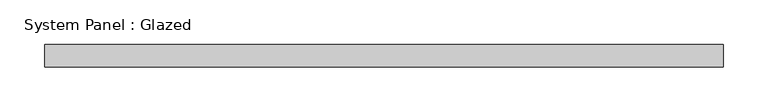
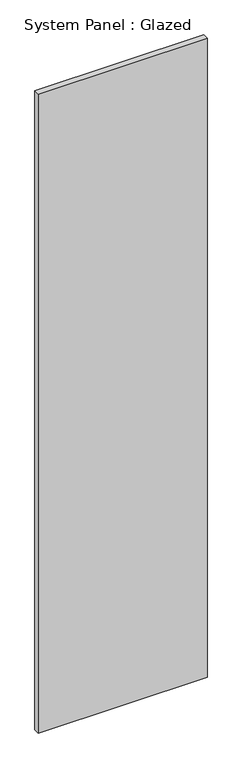
"""IFC4 building model written with IfcOpenShell, lengths in millimetres: plate geometry, System Panel : Glazed."""

from ifc_helpers import new_model, si_unit, origin, origin_with_axes, place, context, project, spatial, polyline, outline, extrude, source, transform, mapped, element, save


def system_panel_glazed_353c4472(model_context):
    return source(origin(), model_context, "Body", "SweptSolid", [
        extrude(outline(polyline([(381.0, 19.05), (-381.0, 19.05), (-381.0, 44.45), (381.0, 44.45), (381.0, 19.05)])), origin_with_axes(), (0.0, 0.0, 1.0), 3048.0),
    ])


if __name__ == "__main__":
    model = new_model("IFC4")
    model_context = context("Model", 3, world=origin())
    ifc_project = project(units=[si_unit("LENGTHUNIT", "METRE", prefix="MILLI")], contexts=[model_context])
    site = spatial("IfcSite", under=ifc_project)
    building = spatial("IfcBuilding", under=site)
    placement = place(None, origin())
    system_panel_glazed_shape = system_panel_glazed_353c4472(model_context)
    element("IfcPlate", 1, ObjectType="System Panel : Glazed", at=placement, inside=building, context=model_context, shape_type="MappedRepresentation", body=[
        mapped(system_panel_glazed_shape, transform((0.0, 0.0, 0.0), x_axis=(1.0, 0.0, 0.0), y_axis=(0.0, 1.0, 0.0), z_axis=(0.0, 0.0, 1.0))),
    ])
    save(model, "model.ifc")

# Revit data of these elements
# Type "System Panel : Glazed"
#   Construction Type Id = "GSP4R"
#   Analytic Construction = "1/8 in Pilkington single glazing"
#   Visual Light Transmittance = 0.9
#   Solar Heat Gain Coefficient = 0.86
#   Heat Transfer Coefficient (U) = 1.18115 BTU/(h·ft²·°F)
#   Define Thermal Properties by = 1
# Element 1 (IfcPlate, "System Panel : Glazed")
#   Materials on its faces: "Glass"
# Materials
#   "Glass": class "Glass", colour RGB 0 128 192, transparency 0.75, Description = "Soda Lime Glass", Cost = 0
